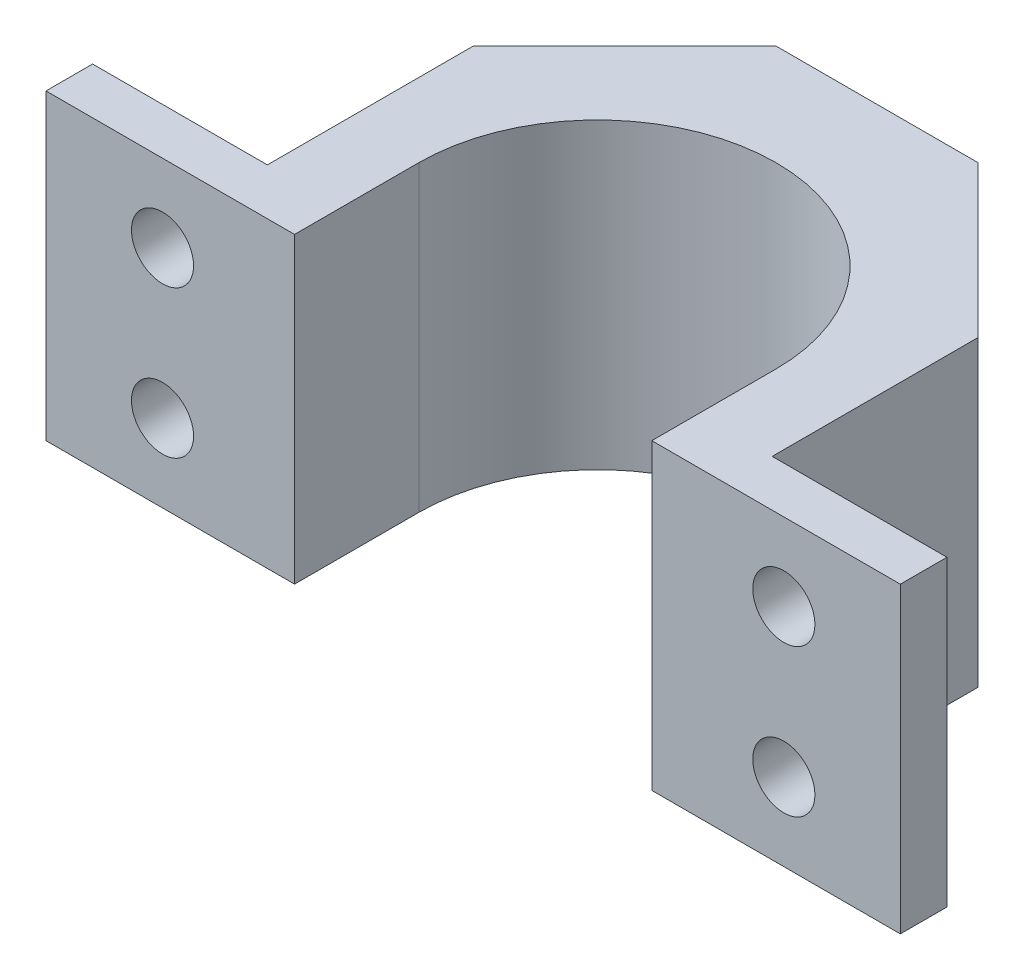
ISO-10303-21;
HEADER;
FILE_DESCRIPTION(('STEP AP214'),'2;1');
FILE_NAME('part.step','',(''),(''),'','','');
FILE_SCHEMA(('AUTOMOTIVE_DESIGN { 1 0 10303 214 1 1 1 1 }'));
ENDSEC;
DATA;
#1=APPLICATION_CONTEXT('core data for automotive mechanical design processes');
#2=APPLICATION_PROTOCOL_DEFINITION('international standard','automotive_design',2000,#1);
#3=PRODUCT_CONTEXT('',#1,'mechanical');
#4=PRODUCT('Part','Part','',(#3));
#5=PRODUCT_RELATED_PRODUCT_CATEGORY('part','',(#4));
#6=PRODUCT_DEFINITION_FORMATION('','',#4);
#7=PRODUCT_DEFINITION_CONTEXT('part definition',#1,'design');
#8=PRODUCT_DEFINITION('design','',#6,#7);
#9=PRODUCT_DEFINITION_SHAPE('','',#8);
#10=(LENGTH_UNIT() NAMED_UNIT(*) SI_UNIT(.MILLI.,.METRE.));
#11=(NAMED_UNIT(*) PLANE_ANGLE_UNIT() SI_UNIT($,.RADIAN.));
#12=(NAMED_UNIT(*) SI_UNIT($,.STERADIAN.) SOLID_ANGLE_UNIT());
#13=UNCERTAINTY_MEASURE_WITH_UNIT(LENGTH_MEASURE(1.E-05),#10,'distance_accuracy_value','');
#14=(GEOMETRIC_REPRESENTATION_CONTEXT(3) GLOBAL_UNCERTAINTY_ASSIGNED_CONTEXT((#13)) GLOBAL_UNIT_ASSIGNED_CONTEXT((#10,
#11,#12)) REPRESENTATION_CONTEXT('',''));
#15=CARTESIAN_POINT('',(0.,0.,0.));
#16=DIRECTION('',(0.,0.,1.));
#17=DIRECTION('',(1.,0.,0.));
#18=AXIS2_PLACEMENT_3D('',#15,#16,#17);
#19=CARTESIAN_POINT('',(0.,0.,6.));
#20=DIRECTION('',(0.,0.,1.));
#21=DIRECTION('',(1.,0.,0.));
#22=AXIS2_PLACEMENT_3D('',#19,#20,#21);
#23=PLANE('',#22);
#24=CARTESIAN_POINT('',(15.,10.,6.));
#25=DIRECTION('',(0.,0.,1.));
#26=DIRECTION('',(1.,0.,0.));
#27=AXIS2_PLACEMENT_3D('',#24,#25,#26);
#28=CIRCLE('',#27,4.);
#29=CARTESIAN_POINT('',(19.,10.,6.));
#30=VERTEX_POINT('',#29);
#31=EDGE_CURVE('E267',#30,#30,#28,.T.);
#32=ORIENTED_EDGE('',*,*,#31,.F.);
#33=EDGE_LOOP('',(#32));
#34=FACE_BOUND('',#33,.T.);
#35=CARTESIAN_POINT('',(15.,29.,6.));
#36=DIRECTION('',(0.,0.,1.));
#37=DIRECTION('',(1.,0.,0.));
#38=AXIS2_PLACEMENT_3D('',#35,#36,#37);
#39=CIRCLE('',#38,4.);
#40=CARTESIAN_POINT('',(19.,29.,6.));
#41=VERTEX_POINT('',#40);
#42=EDGE_CURVE('E213',#41,#41,#39,.T.);
#43=ORIENTED_EDGE('',*,*,#42,.F.);
#44=EDGE_LOOP('',(#43));
#45=FACE_BOUND('',#44,.T.);
#46=DIRECTION('',(0.,-1.,0.));
#47=VECTOR('',#46,1.);
#48=CARTESIAN_POINT('',(32.,39.,6.));
#49=LINE('',#48,#47);
#50=CARTESIAN_POINT('',(32.,39.,6.));
#51=VERTEX_POINT('',#50);
#52=CARTESIAN_POINT('',(32.,0.,6.));
#53=VERTEX_POINT('',#52);
#54=EDGE_CURVE('E179',#51,#53,#49,.T.);
#55=ORIENTED_EDGE('',*,*,#54,.F.);
#56=DIRECTION('',(-1.,0.,0.));
#57=VECTOR('',#56,1.);
#58=CARTESIAN_POINT('',(110.,39.,6.));
#59=LINE('',#58,#57);
#60=CARTESIAN_POINT('',(0.,39.,6.));
#61=VERTEX_POINT('',#60);
#62=EDGE_CURVE('E71',#51,#61,#59,.T.);
#63=ORIENTED_EDGE('',*,*,#62,.T.);
#64=DIRECTION('',(0.,-1.,0.));
#65=VECTOR('',#64,1.);
#66=CARTESIAN_POINT('',(0.,39.,6.));
#67=LINE('',#66,#65);
#68=CARTESIAN_POINT('',(0.,0.,6.));
#69=VERTEX_POINT('',#68);
#70=EDGE_CURVE('E204',#61,#69,#67,.T.);
#71=ORIENTED_EDGE('',*,*,#70,.T.);
#72=DIRECTION('',(1.,0.,0.));
#73=VECTOR('',#72,1.);
#74=CARTESIAN_POINT('',(0.,0.,6.));
#75=LINE('',#74,#73);
#76=EDGE_CURVE('E99',#69,#53,#75,.T.);
#77=ORIENTED_EDGE('',*,*,#76,.T.);
#78=EDGE_LOOP('',(#55,#63,#71,#77));
#79=FACE_BOUND('',#78,.T.);
#80=ADVANCED_FACE('F50',(#34,#45,#79),#23,.T.);
#81=CARTESIAN_POINT('',(0.,0.,0.));
#82=DIRECTION('',(0.,0.,1.));
#83=DIRECTION('',(1.,0.,0.));
#84=AXIS2_PLACEMENT_3D('',#81,#82,#83);
#85=PLANE('',#84);
#86=CARTESIAN_POINT('',(15.,10.,0.));
#87=DIRECTION('',(0.,0.,1.));
#88=DIRECTION('',(1.,0.,0.));
#89=AXIS2_PLACEMENT_3D('',#86,#87,#88);
#90=CIRCLE('',#89,4.);
#91=CARTESIAN_POINT('',(19.,10.,0.));
#92=VERTEX_POINT('',#91);
#93=EDGE_CURVE('E51',#92,#92,#90,.T.);
#94=ORIENTED_EDGE('',*,*,#93,.T.);
#95=EDGE_LOOP('',(#94));
#96=FACE_BOUND('',#95,.T.);
#97=CARTESIAN_POINT('',(15.,29.,0.));
#98=DIRECTION('',(0.,0.,1.));
#99=DIRECTION('',(1.,0.,0.));
#100=AXIS2_PLACEMENT_3D('',#97,#98,#99);
#101=CIRCLE('',#100,4.);
#102=CARTESIAN_POINT('',(19.,29.,0.));
#103=VERTEX_POINT('',#102);
#104=EDGE_CURVE('E214',#103,#103,#101,.T.);
#105=ORIENTED_EDGE('',*,*,#104,.T.);
#106=EDGE_LOOP('',(#105));
#107=FACE_BOUND('',#106,.T.);
#108=DIRECTION('',(0.,-1.,0.));
#109=VECTOR('',#108,1.);
#110=CARTESIAN_POINT('',(22.5,39.,0.));
#111=LINE('',#110,#109);
#112=CARTESIAN_POINT('',(22.5,39.,0.));
#113=VERTEX_POINT('',#112);
#114=CARTESIAN_POINT('',(22.5,0.,0.));
#115=VERTEX_POINT('',#114);
#116=EDGE_CURVE('E317',#113,#115,#111,.T.);
#117=ORIENTED_EDGE('',*,*,#116,.T.);
#118=DIRECTION('',(1.,0.,0.));
#119=VECTOR('',#118,1.);
#120=CARTESIAN_POINT('',(0.,0.,0.));
#121=LINE('',#120,#119);
#122=CARTESIAN_POINT('',(0.,0.,0.));
#123=VERTEX_POINT('',#122);
#124=EDGE_CURVE('E197',#123,#115,#121,.T.);
#125=ORIENTED_EDGE('',*,*,#124,.F.);
#126=DIRECTION('',(0.,-1.,0.));
#127=VECTOR('',#126,1.);
#128=CARTESIAN_POINT('',(0.,39.,0.));
#129=LINE('',#128,#127);
#130=CARTESIAN_POINT('',(0.,39.,0.));
#131=VERTEX_POINT('',#130);
#132=EDGE_CURVE('E195',#131,#123,#129,.T.);
#133=ORIENTED_EDGE('',*,*,#132,.F.);
#134=DIRECTION('',(-1.,0.,0.));
#135=VECTOR('',#134,1.);
#136=CARTESIAN_POINT('',(110.,39.,0.));
#137=LINE('',#136,#135);
#138=EDGE_CURVE('E94',#113,#131,#137,.T.);
#139=ORIENTED_EDGE('',*,*,#138,.F.);
#140=EDGE_LOOP('',(#117,#125,#133,#139));
#141=FACE_BOUND('',#140,.T.);
#142=ADVANCED_FACE('F225',(#96,#107,#141),#85,.F.);
#143=CARTESIAN_POINT('',(0.,39.,6.));
#144=DIRECTION('',(1.,0.,0.));
#145=DIRECTION('',(0.,0.,-1.));
#146=AXIS2_PLACEMENT_3D('',#143,#144,#145);
#147=PLANE('',#146);
#148=ORIENTED_EDGE('',*,*,#132,.T.);
#149=DIRECTION('',(0.,0.,-1.));
#150=VECTOR('',#149,1.);
#151=CARTESIAN_POINT('',(0.,0.,6.));
#152=LINE('',#151,#150);
#153=EDGE_CURVE('E11',#69,#123,#152,.T.);
#154=ORIENTED_EDGE('',*,*,#153,.F.);
#155=ORIENTED_EDGE('',*,*,#70,.F.);
#156=DIRECTION('',(0.,0.,-1.));
#157=VECTOR('',#156,1.);
#158=CARTESIAN_POINT('',(0.,39.,6.));
#159=LINE('',#158,#157);
#160=EDGE_CURVE('E183',#61,#131,#159,.T.);
#161=ORIENTED_EDGE('',*,*,#160,.T.);
#162=EDGE_LOOP('',(#148,#154,#155,#161));
#163=FACE_BOUND('',#162,.T.);
#164=ADVANCED_FACE('F47',(#163),#147,.F.);
#165=CARTESIAN_POINT('',(0.,0.,6.));
#166=DIRECTION('',(0.,1.,0.));
#167=DIRECTION('',(0.,0.,1.));
#168=AXIS2_PLACEMENT_3D('',#165,#166,#167);
#169=PLANE('',#168);
#170=DIRECTION('',(0.,0.,1.));
#171=VECTOR('',#170,1.);
#172=CARTESIAN_POINT('',(32.,0.,0.));
#173=LINE('',#172,#171);
#174=CARTESIAN_POINT('',(32.,0.,-9.99999999999999));
#175=VERTEX_POINT('',#174);
#176=EDGE_CURVE('E294',#175,#53,#173,.T.);
#177=ORIENTED_EDGE('',*,*,#176,.T.);
#178=ORIENTED_EDGE('',*,*,#76,.F.);
#179=ORIENTED_EDGE('',*,*,#153,.T.);
#180=ORIENTED_EDGE('',*,*,#124,.T.);
#181=DIRECTION('',(0.,0.,1.));
#182=VECTOR('',#181,1.);
#183=CARTESIAN_POINT('',(22.5,0.,0.));
#184=LINE('',#183,#182);
#185=CARTESIAN_POINT('',(22.5,0.,-26.5000000000002));
#186=VERTEX_POINT('',#185);
#187=EDGE_CURVE('E299',#186,#115,#184,.T.);
#188=ORIENTED_EDGE('',*,*,#187,.F.);
#189=DIRECTION('',(-0.707106781186551,0.,0.707106781186544));
#190=VECTOR('',#189,1.);
#191=CARTESIAN_POINT('',(-2.00000000000022,0.,-2.00000000000024));
#192=LINE('',#191,#190);
#193=CARTESIAN_POINT('',(42.,0.,-46.));
#194=VERTEX_POINT('',#193);
#195=EDGE_CURVE('E300',#194,#186,#192,.T.);
#196=ORIENTED_EDGE('',*,*,#195,.F.);
#197=DIRECTION('',(1.,0.,0.));
#198=VECTOR('',#197,1.);
#199=CARTESIAN_POINT('',(0.,0.,-46.));
#200=LINE('',#199,#198);
#201=CARTESIAN_POINT('',(68.,0.,-46.));
#202=VERTEX_POINT('',#201);
#203=EDGE_CURVE('E297',#194,#202,#200,.T.);
#204=ORIENTED_EDGE('',*,*,#203,.T.);
#205=DIRECTION('',(0.707106781186546,0.,0.707106781186549));
#206=VECTOR('',#205,1.);
#207=CARTESIAN_POINT('',(57.0000000000002,0.,-56.9999999999999));
#208=LINE('',#207,#206);
#209=CARTESIAN_POINT('',(87.5,0.,-26.4999999999999));
#210=VERTEX_POINT('',#209);
#211=EDGE_CURVE('E301',#202,#210,#208,.T.);
#212=ORIENTED_EDGE('',*,*,#211,.T.);
#213=DIRECTION('',(0.,0.,1.));
#214=VECTOR('',#213,1.);
#215=CARTESIAN_POINT('',(87.5,0.,0.));
#216=LINE('',#215,#214);
#217=CARTESIAN_POINT('',(87.5,0.,0.));
#218=VERTEX_POINT('',#217);
#219=EDGE_CURVE('E63',#210,#218,#216,.T.);
#220=ORIENTED_EDGE('',*,*,#219,.T.);
#221=CARTESIAN_POINT('',(110.,0.,0.));
#222=VERTEX_POINT('',#221);
#223=EDGE_CURVE('E192',#218,#222,#121,.T.);
#224=ORIENTED_EDGE('',*,*,#223,.T.);
#225=DIRECTION('',(0.,0.,-1.));
#226=VECTOR('',#225,1.);
#227=CARTESIAN_POINT('',(110.,0.,6.));
#228=LINE('',#227,#226);
#229=CARTESIAN_POINT('',(110.,0.,6.));
#230=VERTEX_POINT('',#229);
#231=EDGE_CURVE('E57',#230,#222,#228,.T.);
#232=ORIENTED_EDGE('',*,*,#231,.F.);
#233=CARTESIAN_POINT('',(78.,0.,6.));
#234=VERTEX_POINT('',#233);
#235=EDGE_CURVE('E323',#234,#230,#75,.T.);
#236=ORIENTED_EDGE('',*,*,#235,.F.);
#237=DIRECTION('',(0.,0.,1.));
#238=VECTOR('',#237,1.);
#239=CARTESIAN_POINT('',(78.,0.,0.));
#240=LINE('',#239,#238);
#241=CARTESIAN_POINT('',(78.,0.,-9.99999999999999));
#242=VERTEX_POINT('',#241);
#243=EDGE_CURVE('E178',#242,#234,#240,.T.);
#244=ORIENTED_EDGE('',*,*,#243,.F.);
#245=CARTESIAN_POINT('',(55.,0.,-9.99999999999999));
#246=DIRECTION('',(0.,-1.,0.));
#247=DIRECTION('',(0.,0.,-1.));
#248=AXIS2_PLACEMENT_3D('',#245,#246,#247);
#249=CIRCLE('',#248,23.);
#250=EDGE_CURVE('E277',#175,#242,#249,.T.);
#251=ORIENTED_EDGE('',*,*,#250,.F.);
#252=EDGE_LOOP('',(#177,#178,#179,#180,#188,#196,#204,#212,#220,#224,#232,#236,#244,#251));
#253=FACE_BOUND('',#252,.T.);
#254=ADVANCED_FACE('F324',(#253),#169,.F.);
#255=CARTESIAN_POINT('',(110.,0.,6.));
#256=DIRECTION('',(-1.,0.,0.));
#257=DIRECTION('',(0.,0.,1.));
#258=AXIS2_PLACEMENT_3D('',#255,#256,#257);
#259=PLANE('',#258);
#260=DIRECTION('',(0.,1.,0.));
#261=VECTOR('',#260,1.);
#262=CARTESIAN_POINT('',(110.,0.,0.));
#263=LINE('',#262,#261);
#264=CARTESIAN_POINT('',(110.,39.,0.));
#265=VERTEX_POINT('',#264);
#266=EDGE_CURVE('E199',#222,#265,#263,.T.);
#267=ORIENTED_EDGE('',*,*,#266,.T.);
#268=DIRECTION('',(0.,0.,-1.));
#269=VECTOR('',#268,1.);
#270=CARTESIAN_POINT('',(110.,39.,6.));
#271=LINE('',#270,#269);
#272=CARTESIAN_POINT('',(110.,39.,6.));
#273=VERTEX_POINT('',#272);
#274=EDGE_CURVE('E186',#273,#265,#271,.T.);
#275=ORIENTED_EDGE('',*,*,#274,.F.);
#276=DIRECTION('',(0.,1.,0.));
#277=VECTOR('',#276,1.);
#278=CARTESIAN_POINT('',(110.,0.,6.));
#279=LINE('',#278,#277);
#280=EDGE_CURVE('E181',#230,#273,#279,.T.);
#281=ORIENTED_EDGE('',*,*,#280,.F.);
#282=ORIENTED_EDGE('',*,*,#231,.T.);
#283=EDGE_LOOP('',(#267,#275,#281,#282));
#284=FACE_BOUND('',#283,.T.);
#285=ADVANCED_FACE('F256',(#284),#259,.F.);
#286=CARTESIAN_POINT('',(110.,39.,6.));
#287=DIRECTION('',(0.,-1.,0.));
#288=DIRECTION('',(0.,0.,-1.));
#289=AXIS2_PLACEMENT_3D('',#286,#287,#288);
#290=PLANE('',#289);
#291=ORIENTED_EDGE('',*,*,#62,.F.);
#292=DIRECTION('',(0.,0.,1.));
#293=VECTOR('',#292,1.);
#294=CARTESIAN_POINT('',(32.,39.,0.));
#295=LINE('',#294,#293);
#296=CARTESIAN_POINT('',(32.,39.,-9.99999999999999));
#297=VERTEX_POINT('',#296);
#298=EDGE_CURVE('E276',#297,#51,#295,.T.);
#299=ORIENTED_EDGE('',*,*,#298,.F.);
#300=CARTESIAN_POINT('',(55.,39.,-9.99999999999999));
#301=DIRECTION('',(0.,-1.,0.));
#302=DIRECTION('',(0.,0.,-1.));
#303=AXIS2_PLACEMENT_3D('',#300,#301,#302);
#304=CIRCLE('',#303,23.);
#305=CARTESIAN_POINT('',(78.,39.,-9.99999999999999));
#306=VERTEX_POINT('',#305);
#307=EDGE_CURVE('E167',#297,#306,#304,.T.);
#308=ORIENTED_EDGE('',*,*,#307,.T.);
#309=DIRECTION('',(0.,0.,1.));
#310=VECTOR('',#309,1.);
#311=CARTESIAN_POINT('',(78.,39.,0.));
#312=LINE('',#311,#310);
#313=CARTESIAN_POINT('',(78.,39.,6.));
#314=VERTEX_POINT('',#313);
#315=EDGE_CURVE('E158',#306,#314,#312,.T.);
#316=ORIENTED_EDGE('',*,*,#315,.T.);
#317=EDGE_CURVE('E162',#273,#314,#59,.T.);
#318=ORIENTED_EDGE('',*,*,#317,.F.);
#319=ORIENTED_EDGE('',*,*,#274,.T.);
#320=CARTESIAN_POINT('',(87.5,39.,0.));
#321=VERTEX_POINT('',#320);
#322=EDGE_CURVE('E205',#265,#321,#137,.T.);
#323=ORIENTED_EDGE('',*,*,#322,.T.);
#324=DIRECTION('',(0.,0.,1.));
#325=VECTOR('',#324,1.);
#326=CARTESIAN_POINT('',(87.5,39.,0.));
#327=LINE('',#326,#325);
#328=CARTESIAN_POINT('',(87.5,39.,-26.4999999999999));
#329=VERTEX_POINT('',#328);
#330=EDGE_CURVE('E174',#329,#321,#327,.T.);
#331=ORIENTED_EDGE('',*,*,#330,.F.);
#332=DIRECTION('',(0.707106781186546,0.,0.707106781186549));
#333=VECTOR('',#332,1.);
#334=CARTESIAN_POINT('',(57.0000000000002,39.,-56.9999999999999));
#335=LINE('',#334,#333);
#336=CARTESIAN_POINT('',(68.,39.,-46.));
#337=VERTEX_POINT('',#336);
#338=EDGE_CURVE('E286',#337,#329,#335,.T.);
#339=ORIENTED_EDGE('',*,*,#338,.F.);
#340=DIRECTION('',(1.,0.,0.));
#341=VECTOR('',#340,1.);
#342=CARTESIAN_POINT('',(0.,39.,-46.));
#343=LINE('',#342,#341);
#344=CARTESIAN_POINT('',(42.,39.,-46.));
#345=VERTEX_POINT('',#344);
#346=EDGE_CURVE('E282',#345,#337,#343,.T.);
#347=ORIENTED_EDGE('',*,*,#346,.F.);
#348=DIRECTION('',(-0.707106781186551,0.,0.707106781186544));
#349=VECTOR('',#348,1.);
#350=CARTESIAN_POINT('',(-2.00000000000022,39.,-2.00000000000024));
#351=LINE('',#350,#349);
#352=CARTESIAN_POINT('',(22.5,39.,-26.5000000000002));
#353=VERTEX_POINT('',#352);
#354=EDGE_CURVE('E285',#345,#353,#351,.T.);
#355=ORIENTED_EDGE('',*,*,#354,.T.);
#356=DIRECTION('',(0.,0.,1.));
#357=VECTOR('',#356,1.);
#358=CARTESIAN_POINT('',(22.5,39.,0.));
#359=LINE('',#358,#357);
#360=EDGE_CURVE('E284',#353,#113,#359,.T.);
#361=ORIENTED_EDGE('',*,*,#360,.T.);
#362=ORIENTED_EDGE('',*,*,#138,.T.);
#363=ORIENTED_EDGE('',*,*,#160,.F.);
#364=EDGE_LOOP('',(#291,#299,#308,#316,#318,#319,#323,#331,#339,#347,#355,#361,#362,#363));
#365=FACE_BOUND('',#364,.T.);
#366=ADVANCED_FACE('F159',(#365),#290,.F.);
#367=CARTESIAN_POINT('',(95.,29.,6.));
#368=DIRECTION('',(0.,0.,1.));
#369=DIRECTION('',(1.,0.,0.));
#370=AXIS2_PLACEMENT_3D('',#367,#368,#369);
#371=CIRCLE('',#370,4.00000000000001);
#372=CARTESIAN_POINT('',(99.,29.,6.));
#373=VERTEX_POINT('',#372);
#374=EDGE_CURVE('E263',#373,#373,#371,.T.);
#375=ORIENTED_EDGE('',*,*,#374,.F.);
#376=EDGE_LOOP('',(#375));
#377=FACE_BOUND('',#376,.T.);
#378=CARTESIAN_POINT('',(95.,10.,6.));
#379=DIRECTION('',(0.,0.,1.));
#380=DIRECTION('',(1.,0.,0.));
#381=AXIS2_PLACEMENT_3D('',#378,#379,#380);
#382=CIRCLE('',#381,4.00000000000001);
#383=CARTESIAN_POINT('',(99.,10.,6.));
#384=VERTEX_POINT('',#383);
#385=EDGE_CURVE('E266',#384,#384,#382,.T.);
#386=ORIENTED_EDGE('',*,*,#385,.F.);
#387=EDGE_LOOP('',(#386));
#388=FACE_BOUND('',#387,.T.);
#389=DIRECTION('',(0.,-1.,0.));
#390=VECTOR('',#389,1.);
#391=CARTESIAN_POINT('',(78.,39.,6.));
#392=LINE('',#391,#390);
#393=EDGE_CURVE('E173',#314,#234,#392,.T.);
#394=ORIENTED_EDGE('',*,*,#393,.T.);
#395=ORIENTED_EDGE('',*,*,#235,.T.);
#396=ORIENTED_EDGE('',*,*,#280,.T.);
#397=ORIENTED_EDGE('',*,*,#317,.T.);
#398=EDGE_LOOP('',(#394,#395,#396,#397));
#399=FACE_BOUND('',#398,.T.);
#400=ADVANCED_FACE('F182',(#377,#388,#399),#23,.T.);
#401=CARTESIAN_POINT('',(95.,29.,0.));
#402=DIRECTION('',(0.,0.,1.));
#403=DIRECTION('',(1.,0.,0.));
#404=AXIS2_PLACEMENT_3D('',#401,#402,#403);
#405=CIRCLE('',#404,4.00000000000001);
#406=CARTESIAN_POINT('',(99.,29.,0.));
#407=VERTEX_POINT('',#406);
#408=EDGE_CURVE('E215',#407,#407,#405,.T.);
#409=ORIENTED_EDGE('',*,*,#408,.T.);
#410=EDGE_LOOP('',(#409));
#411=FACE_BOUND('',#410,.T.);
#412=CARTESIAN_POINT('',(95.,10.,0.));
#413=DIRECTION('',(0.,0.,1.));
#414=DIRECTION('',(1.,0.,0.));
#415=AXIS2_PLACEMENT_3D('',#412,#413,#414);
#416=CIRCLE('',#415,4.00000000000001);
#417=CARTESIAN_POINT('',(99.,10.,0.));
#418=VERTEX_POINT('',#417);
#419=EDGE_CURVE('E207',#418,#418,#416,.T.);
#420=ORIENTED_EDGE('',*,*,#419,.T.);
#421=EDGE_LOOP('',(#420));
#422=FACE_BOUND('',#421,.T.);
#423=ORIENTED_EDGE('',*,*,#223,.F.);
#424=DIRECTION('',(0.,-1.,0.));
#425=VECTOR('',#424,1.);
#426=CARTESIAN_POINT('',(87.5,39.,0.));
#427=LINE('',#426,#425);
#428=EDGE_CURVE('E306',#321,#218,#427,.T.);
#429=ORIENTED_EDGE('',*,*,#428,.F.);
#430=ORIENTED_EDGE('',*,*,#322,.F.);
#431=ORIENTED_EDGE('',*,*,#266,.F.);
#432=EDGE_LOOP('',(#423,#429,#430,#431));
#433=FACE_BOUND('',#432,.T.);
#434=ADVANCED_FACE('F248',(#411,#422,#433),#85,.F.);
#435=CARTESIAN_POINT('',(55.,39.,-9.99999999999999));
#436=DIRECTION('',(0.,-1.,0.));
#437=DIRECTION('',(0.,0.,-1.));
#438=AXIS2_PLACEMENT_3D('',#435,#436,#437);
#439=CYLINDRICAL_SURFACE('',#438,23.);
#440=ORIENTED_EDGE('',*,*,#250,.T.);
#441=DIRECTION('',(0.,-1.,0.));
#442=VECTOR('',#441,1.);
#443=CARTESIAN_POINT('',(78.,39.,-9.99999999999999));
#444=LINE('',#443,#442);
#445=EDGE_CURVE('E198',#306,#242,#444,.T.);
#446=ORIENTED_EDGE('',*,*,#445,.F.);
#447=ORIENTED_EDGE('',*,*,#307,.F.);
#448=DIRECTION('',(0.,-1.,0.));
#449=VECTOR('',#448,1.);
#450=CARTESIAN_POINT('',(32.,39.,-9.99999999999999));
#451=LINE('',#450,#449);
#452=EDGE_CURVE('E168',#297,#175,#451,.T.);
#453=ORIENTED_EDGE('',*,*,#452,.T.);
#454=EDGE_LOOP('',(#440,#446,#447,#453));
#455=FACE_BOUND('',#454,.T.);
#456=ADVANCED_FACE('F254',(#455),#439,.F.);
#457=CARTESIAN_POINT('',(78.,39.,0.));
#458=DIRECTION('',(1.,0.,0.));
#459=DIRECTION('',(0.,0.,-1.));
#460=AXIS2_PLACEMENT_3D('',#457,#458,#459);
#461=PLANE('',#460);
#462=ORIENTED_EDGE('',*,*,#243,.T.);
#463=ORIENTED_EDGE('',*,*,#393,.F.);
#464=ORIENTED_EDGE('',*,*,#315,.F.);
#465=ORIENTED_EDGE('',*,*,#445,.T.);
#466=EDGE_LOOP('',(#462,#463,#464,#465));
#467=FACE_BOUND('',#466,.T.);
#468=ADVANCED_FACE('F172',(#467),#461,.F.);
#469=CARTESIAN_POINT('',(87.5,39.,0.));
#470=DIRECTION('',(1.,0.,0.));
#471=DIRECTION('',(0.,0.,-1.));
#472=AXIS2_PLACEMENT_3D('',#469,#470,#471);
#473=PLANE('',#472);
#474=ORIENTED_EDGE('',*,*,#219,.F.);
#475=DIRECTION('',(0.,-1.,0.));
#476=VECTOR('',#475,1.);
#477=CARTESIAN_POINT('',(87.5,39.,-26.4999999999999));
#478=LINE('',#477,#476);
#479=EDGE_CURVE('E309',#329,#210,#478,.T.);
#480=ORIENTED_EDGE('',*,*,#479,.F.);
#481=ORIENTED_EDGE('',*,*,#330,.T.);
#482=ORIENTED_EDGE('',*,*,#428,.T.);
#483=EDGE_LOOP('',(#474,#480,#481,#482));
#484=FACE_BOUND('',#483,.T.);
#485=ADVANCED_FACE('F331',(#484),#473,.T.);
#486=CARTESIAN_POINT('',(57.0000000000002,39.,-56.9999999999999));
#487=DIRECTION('',(0.707106781186549,0.,-0.707106781186546));
#488=DIRECTION('',(-0.707106781186546,0.,-0.707106781186549));
#489=AXIS2_PLACEMENT_3D('',#486,#487,#488);
#490=PLANE('',#489);
#491=ORIENTED_EDGE('',*,*,#211,.F.);
#492=DIRECTION('',(0.,-1.,0.));
#493=VECTOR('',#492,1.);
#494=CARTESIAN_POINT('',(68.,39.,-46.));
#495=LINE('',#494,#493);
#496=EDGE_CURVE('E315',#337,#202,#495,.T.);
#497=ORIENTED_EDGE('',*,*,#496,.F.);
#498=ORIENTED_EDGE('',*,*,#338,.T.);
#499=ORIENTED_EDGE('',*,*,#479,.T.);
#500=EDGE_LOOP('',(#491,#497,#498,#499));
#501=FACE_BOUND('',#500,.T.);
#502=ADVANCED_FACE('F338',(#501),#490,.T.);
#503=CARTESIAN_POINT('',(0.,39.,-46.));
#504=DIRECTION('',(0.,0.,-1.));
#505=DIRECTION('',(-1.,0.,0.));
#506=AXIS2_PLACEMENT_3D('',#503,#504,#505);
#507=PLANE('',#506);
#508=ORIENTED_EDGE('',*,*,#203,.F.);
#509=DIRECTION('',(0.,-1.,0.));
#510=VECTOR('',#509,1.);
#511=CARTESIAN_POINT('',(42.,39.,-46.));
#512=LINE('',#511,#510);
#513=EDGE_CURVE('E314',#345,#194,#512,.T.);
#514=ORIENTED_EDGE('',*,*,#513,.F.);
#515=ORIENTED_EDGE('',*,*,#346,.T.);
#516=ORIENTED_EDGE('',*,*,#496,.T.);
#517=EDGE_LOOP('',(#508,#514,#515,#516));
#518=FACE_BOUND('',#517,.T.);
#519=ADVANCED_FACE('F345',(#518),#507,.T.);
#520=CARTESIAN_POINT('',(-2.00000000000022,39.,-2.00000000000024));
#521=DIRECTION('',(0.707106781186544,0.,0.707106781186551));
#522=DIRECTION('',(0.707106781186551,0.,-0.707106781186544));
#523=AXIS2_PLACEMENT_3D('',#520,#521,#522);
#524=PLANE('',#523);
#525=ORIENTED_EDGE('',*,*,#195,.T.);
#526=DIRECTION('',(0.,-1.,0.));
#527=VECTOR('',#526,1.);
#528=CARTESIAN_POINT('',(22.5,39.,-26.5000000000002));
#529=LINE('',#528,#527);
#530=EDGE_CURVE('E316',#353,#186,#529,.T.);
#531=ORIENTED_EDGE('',*,*,#530,.F.);
#532=ORIENTED_EDGE('',*,*,#354,.F.);
#533=ORIENTED_EDGE('',*,*,#513,.T.);
#534=EDGE_LOOP('',(#525,#531,#532,#533));
#535=FACE_BOUND('',#534,.T.);
#536=ADVANCED_FACE('F346',(#535),#524,.F.);
#537=CARTESIAN_POINT('',(22.5,39.,0.));
#538=DIRECTION('',(1.,0.,0.));
#539=DIRECTION('',(0.,0.,-1.));
#540=AXIS2_PLACEMENT_3D('',#537,#538,#539);
#541=PLANE('',#540);
#542=ORIENTED_EDGE('',*,*,#187,.T.);
#543=ORIENTED_EDGE('',*,*,#116,.F.);
#544=ORIENTED_EDGE('',*,*,#360,.F.);
#545=ORIENTED_EDGE('',*,*,#530,.T.);
#546=EDGE_LOOP('',(#542,#543,#544,#545));
#547=FACE_BOUND('',#546,.T.);
#548=ADVANCED_FACE('F351',(#547),#541,.F.);
#549=CARTESIAN_POINT('',(32.,39.,0.));
#550=DIRECTION('',(1.,0.,0.));
#551=DIRECTION('',(0.,0.,-1.));
#552=AXIS2_PLACEMENT_3D('',#549,#550,#551);
#553=PLANE('',#552);
#554=ORIENTED_EDGE('',*,*,#176,.F.);
#555=ORIENTED_EDGE('',*,*,#452,.F.);
#556=ORIENTED_EDGE('',*,*,#298,.T.);
#557=ORIENTED_EDGE('',*,*,#54,.T.);
#558=EDGE_LOOP('',(#554,#555,#556,#557));
#559=FACE_BOUND('',#558,.T.);
#560=ADVANCED_FACE('F357',(#559),#553,.T.);
#561=CARTESIAN_POINT('',(95.,10.,-33.));
#562=DIRECTION('',(0.,0.,1.));
#563=DIRECTION('',(1.,0.,0.));
#564=AXIS2_PLACEMENT_3D('',#561,#562,#563);
#565=CYLINDRICAL_SURFACE('',#564,4.00000000000001);
#566=ORIENTED_EDGE('',*,*,#385,.T.);
#567=EDGE_LOOP('',(#566));
#568=FACE_BOUND('',#567,.T.);
#569=ORIENTED_EDGE('',*,*,#419,.F.);
#570=EDGE_LOOP('',(#569));
#571=FACE_BOUND('',#570,.T.);
#572=ADVANCED_FACE('F371',(#568,#571),#565,.F.);
#573=CARTESIAN_POINT('',(95.,29.,-33.));
#574=DIRECTION('',(0.,0.,1.));
#575=DIRECTION('',(1.,0.,0.));
#576=AXIS2_PLACEMENT_3D('',#573,#574,#575);
#577=CYLINDRICAL_SURFACE('',#576,4.00000000000001);
#578=ORIENTED_EDGE('',*,*,#374,.T.);
#579=EDGE_LOOP('',(#578));
#580=FACE_BOUND('',#579,.T.);
#581=ORIENTED_EDGE('',*,*,#408,.F.);
#582=EDGE_LOOP('',(#581));
#583=FACE_BOUND('',#582,.T.);
#584=ADVANCED_FACE('F235',(#580,#583),#577,.F.);
#585=CARTESIAN_POINT('',(15.,29.,-33.));
#586=DIRECTION('',(0.,0.,1.));
#587=DIRECTION('',(1.,0.,0.));
#588=AXIS2_PLACEMENT_3D('',#585,#586,#587);
#589=CYLINDRICAL_SURFACE('',#588,4.);
#590=ORIENTED_EDGE('',*,*,#42,.T.);
#591=EDGE_LOOP('',(#590));
#592=FACE_BOUND('',#591,.T.);
#593=ORIENTED_EDGE('',*,*,#104,.F.);
#594=EDGE_LOOP('',(#593));
#595=FACE_BOUND('',#594,.T.);
#596=ADVANCED_FACE('F229',(#592,#595),#589,.F.);
#597=CARTESIAN_POINT('',(15.,10.,-33.));
#598=DIRECTION('',(0.,0.,1.));
#599=DIRECTION('',(1.,0.,0.));
#600=AXIS2_PLACEMENT_3D('',#597,#598,#599);
#601=CYLINDRICAL_SURFACE('',#600,4.);
#602=ORIENTED_EDGE('',*,*,#31,.T.);
#603=EDGE_LOOP('',(#602));
#604=FACE_BOUND('',#603,.T.);
#605=ORIENTED_EDGE('',*,*,#93,.F.);
#606=EDGE_LOOP('',(#605));
#607=FACE_BOUND('',#606,.T.);
#608=ADVANCED_FACE('F221',(#604,#607),#601,.F.);
#609=CLOSED_SHELL('',(#80,#142,#164,#254,#285,#366,#400,#434,#456,#468,#485,#502,#519,#536,#548,
#560,#572,#584,#596,#608));
#610=MANIFOLD_SOLID_BREP('B2',#609);
#611=ADVANCED_BREP_SHAPE_REPRESENTATION('',(#18,#610),#14);
#612=SHAPE_DEFINITION_REPRESENTATION(#9,#611);
ENDSEC;
END-ISO-10303-21;
